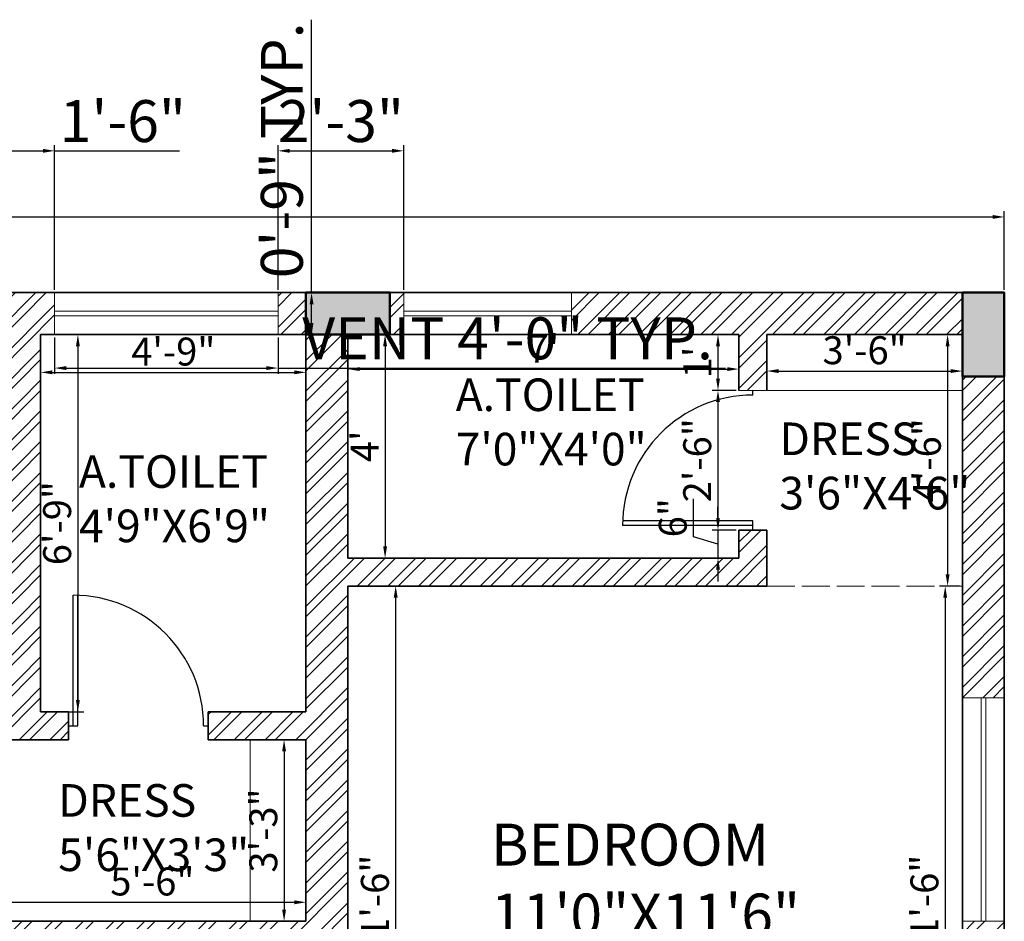
# Model space of a CAD drawing. Units: inches. Extents: x 4153 to 5577, y 785 to 1503.
# Tile 11 of 11: x 5307 to 5518, y 1309 to 1503. Entities that reach past the tile are written whole.
import ezdxf

# ---------------------------------------------------------------- set-up
doc = ezdxf.new("R2010")
doc.units = ezdxf.units.IN
doc.linetypes.add('ACAD_ISO02W100', pattern=[15, 12, -3])
for name, color, linetype, lineweight in [('A-ANNO-DIMS', 2, 'Continuous', 18), ('A-AREA-IDEN', 7, 'Continuous', 25), ('A-COLS', 7, 'Continuous', 50), ('A-DOOR', 3, 'Continuous', 25), ('A-FLOR-CASE', 32, 'Continuous', 18), ('A-GLAZ', 4, 'Continuous', 18), ('A-WALL', 7, 'Continuous', 35), ('A-WALL-OVHD', 7, 'ACAD_ISO02W100', 18)]:
    doc.layers.add(name, color=color, linetype=linetype, lineweight=lineweight)
doc.layers.add('A-WALL-PATT', color=251, linetype='Continuous', lineweight=13, true_color=0x636466)
doc.styles.get("Standard").update_dxf_attribs({"font": 'arial.ttf'})
doc.dimstyles.new('ISO-25', dxfattribs={"dimtxt": 9, "dimasz": 2.5, "dimexe": 1.25, "dimexo": 0.625, "dimtad": 1, "dimlunit": 3, "dimtxsty": 'Standard', "dimcen": 2.5, "dimadec": 0, "dimazin": 0, "dimtfac": 1, "dimtmove": 0, "dimatfit": 3, "dimfxl": 1, "dimarcsym": 0})

# ---------------------------------------------------------------- blocks, each defined once
blk = doc.blocks.new('D2')
for p, q in [((1, 0), (1, 28)), ((2, 0), (2, 27.98)), ((0, 0), (2, 0)), ((29, 0), (30, 0))]:
    blk.add_line(p, q)
at = {"ltscale": 0.5}
blk.add_arc((1, 0), 28, 0, 90, dxfattribs=at)
blk = doc.blocks.new('*D23')
at = {"layer": 'A-ANNO-DIMS', "color": 0, "lineweight": -2, "transparency": 16777216}
for p, q in [((5011.25, 1445.11), (5011.25, 1461.99)), ((5518.25, 1445.11), (5518.25, 1461.99)), ((5013.75, 1460.74), (5515.75, 1460.74))]:
    blk.add_line(p, q, dxfattribs=at)
at = {"layer": 'A-ANNO-DIMS', "color": 0, "transparency": 16777216}
for points in [[(5013.75, 1461.16), (5013.75, 1460.33), (5011.25, 1460.74)], [(5515.75, 1461.16), (5515.75, 1460.33), (5518.25, 1460.74)]]:
    blk.add_solid(points, dxfattribs=at)
at = {"layer": 'Defpoints', "color": 0, "transparency": 16777216}
for p in [(5518.25, 1460.74), (5011.25, 1444.49), (5518.25, 1444.49)]:
    blk.add_point(p, dxfattribs=at)
at = {"layer": 'A-ANNO-DIMS', "color": 0, "transparency": 16777216, "insert": (5264.75, 1465.97), "char_height": 9, "attachment_point": 5}
blk.add_mtext('42\'-3"', dxfattribs=at)
blk = doc.blocks.new('*D67')
at = {"layer": 'A-ANNO-DIMS', "color": 0, "lineweight": -2, "transparency": 16777216}
for p, q in [((5377.88, 1381.49), (5388.77, 1381.49)), ((5387.52, 1245.99), (5387.52, 1378.99)), ((5377.88, 1243.49), (5388.77, 1243.49))]:
    blk.add_line(p, q, dxfattribs=at)
at = {"layer": 'A-ANNO-DIMS', "color": 0, "transparency": 16777216}
for points in [[(5387.1, 1378.99), (5387.94, 1378.99), (5387.52, 1381.49)], [(5387.1, 1245.99), (5387.94, 1245.99), (5387.52, 1243.49)]]:
    blk.add_solid(points, dxfattribs=at)
at = {"layer": 'Defpoints', "color": 0, "transparency": 16777216}
for p in [(5377.25, 1381.49), (5387.52, 1381.49), (5377.25, 1243.49)]:
    blk.add_point(p, dxfattribs=at)
at = {"layer": 'A-ANNO-DIMS', "color": 0, "transparency": 16777216, "insert": (5383.83, 1312.49), "char_height": 6, "attachment_point": 5, "rotation": 90}
blk.add_mtext('11\'-6"', dxfattribs=at)
blk = doc.blocks.new('*D71')
at = {"layer": 'A-ANNO-DIMS', "color": 0, "lineweight": -2, "transparency": 16777216}
for p, q in [((5311.25, 1434.86), (5311.25, 1426.12)), ((5368.25, 1434.86), (5368.25, 1426.12)), ((5313.75, 1427.37), (5365.75, 1427.37))]:
    blk.add_line(p, q, dxfattribs=at)
at = {"layer": 'A-ANNO-DIMS', "color": 0, "transparency": 16777216}
for points in [[(5313.75, 1427.79), (5313.75, 1426.96), (5311.25, 1427.37)], [(5365.75, 1427.79), (5365.75, 1426.96), (5368.25, 1427.37)]]:
    blk.add_solid(points, dxfattribs=at)
at = {"layer": 'Defpoints', "color": 0, "transparency": 16777216}
for p in [(5311.25, 1435.49), (5368.25, 1435.49), (5368.25, 1427.37)]:
    blk.add_point(p, dxfattribs=at)
at = {"layer": 'A-ANNO-DIMS', "color": 0, "transparency": 16777216, "insert": (5339.75, 1431.06), "char_height": 6, "attachment_point": 5}
blk.add_mtext('4\'-9"', dxfattribs=at)
blk = doc.blocks.new('*D72')
at = {"layer": 'A-ANNO-DIMS', "color": 0, "lineweight": -2, "transparency": 16777216}
for p, q in [((5311.88, 1435.49), (5320.5, 1435.49)), ((5319.25, 1432.99), (5319.25, 1356.99)), ((5311.88, 1354.49), (5320.5, 1354.49))]:
    blk.add_line(p, q, dxfattribs=at)
at = {"layer": 'A-ANNO-DIMS', "color": 0, "transparency": 16777216}
for points in [[(5318.84, 1432.99), (5319.67, 1432.99), (5319.25, 1435.49)], [(5318.84, 1356.99), (5319.67, 1356.99), (5319.25, 1354.49)]]:
    blk.add_solid(points, dxfattribs=at)
at = {"layer": 'Defpoints', "color": 0, "transparency": 16777216}
for p in [(5311.25, 1435.49), (5311.25, 1354.49), (5319.25, 1354.49)]:
    blk.add_point(p, dxfattribs=at)
at = {"layer": 'A-ANNO-DIMS', "color": 0, "transparency": 16777216, "insert": (5315.57, 1394.99), "char_height": 6, "attachment_point": 5, "rotation": 90}
blk.add_mtext('6\'-9"', dxfattribs=at)
blk = doc.blocks.new('*D73')
at = {"layer": 'A-ANNO-DIMS', "color": 0, "lineweight": -2, "transparency": 16777216}
for p, q in [((5367.63, 1348.49), (5362.3, 1348.49)), ((5363.55, 1345.99), (5363.55, 1311.99)), ((5367.63, 1309.49), (5362.3, 1309.49))]:
    blk.add_line(p, q, dxfattribs=at)
at = {"layer": 'A-ANNO-DIMS', "color": 0, "transparency": 16777216}
for points in [[(5363.13, 1345.99), (5363.96, 1345.99), (5363.55, 1348.49)], [(5363.13, 1311.99), (5363.96, 1311.99), (5363.55, 1309.49)]]:
    blk.add_solid(points, dxfattribs=at)
at = {"layer": 'Defpoints', "color": 0, "transparency": 16777216}
for p in [(5368.25, 1348.49), (5363.55, 1309.49), (5368.25, 1309.49)]:
    blk.add_point(p, dxfattribs=at)
at = {"layer": 'A-ANNO-DIMS', "color": 0, "transparency": 16777216, "insert": (5359.86, 1328.99), "char_height": 6, "attachment_point": 5, "rotation": 90}
blk.add_mtext('3\'-3"', dxfattribs=at)
blk = doc.blocks.new('*D74')
at = {"layer": 'A-ANNO-DIMS', "color": 0, "lineweight": -2, "transparency": 16777216}
for p, q in [((5302.25, 1310.11), (5302.25, 1314.82)), ((5304.75, 1313.57), (5365.75, 1313.57)), ((5368.25, 1310.11), (5368.25, 1314.82))]:
    blk.add_line(p, q, dxfattribs=at)
at = {"layer": 'A-ANNO-DIMS', "color": 0, "transparency": 16777216}
for points in [[(5304.75, 1313.99), (5304.75, 1313.15), (5302.25, 1313.57)], [(5365.75, 1313.99), (5365.75, 1313.15), (5368.25, 1313.57)]]:
    blk.add_solid(points, dxfattribs=at)
at = {"layer": 'Defpoints', "color": 0, "transparency": 16777216}
for p in [(5368.25, 1313.57), (5302.25, 1309.49), (5368.25, 1309.49)]:
    blk.add_point(p, dxfattribs=at)
at = {"layer": 'A-ANNO-DIMS', "color": 0, "transparency": 16777216, "insert": (5335.25, 1317.26), "char_height": 6, "attachment_point": 5}
blk.add_mtext('5\'-6"', dxfattribs=at)
blk = doc.blocks.new('*D75')
at = {"layer": 'A-ANNO-DIMS', "color": 0, "lineweight": -2, "transparency": 16777216}
for p, q in [((5377.88, 1435.49), (5386.49, 1435.49)), ((5385.24, 1432.99), (5385.24, 1389.99)), ((5377.88, 1387.49), (5386.49, 1387.49))]:
    blk.add_line(p, q, dxfattribs=at)
at = {"layer": 'A-ANNO-DIMS', "color": 0, "transparency": 16777216}
for points in [[(5384.83, 1432.99), (5385.66, 1432.99), (5385.24, 1435.49)], [(5384.83, 1389.99), (5385.66, 1389.99), (5385.24, 1387.49)]]:
    blk.add_solid(points, dxfattribs=at)
at = {"layer": 'Defpoints', "color": 0, "transparency": 16777216}
for p in [(5377.25, 1435.49), (5377.25, 1387.49), (5385.24, 1387.49)]:
    blk.add_point(p, dxfattribs=at)
at = {"layer": 'A-ANNO-DIMS', "color": 0, "transparency": 16777216, "insert": (5381.62, 1411.49), "char_height": 6, "attachment_point": 5, "rotation": 90}
blk.add_mtext("4'", dxfattribs=at)
blk = doc.blocks.new('*D76')
at = {"layer": 'A-ANNO-DIMS', "color": 0, "lineweight": -2, "transparency": 16777216}
for p, q in [((5377.25, 1434.86), (5377.25, 1426.82)), ((5461.25, 1434.86), (5461.25, 1426.82)), ((5379.75, 1428.07), (5458.75, 1428.07))]:
    blk.add_line(p, q, dxfattribs=at)
at = {"layer": 'A-ANNO-DIMS', "color": 0, "transparency": 16777216}
for points in [[(5379.75, 1428.49), (5379.75, 1427.66), (5377.25, 1428.07)], [(5458.75, 1428.49), (5458.75, 1427.66), (5461.25, 1428.07)]]:
    blk.add_solid(points, dxfattribs=at)
at = {"layer": 'Defpoints', "color": 0, "transparency": 16777216}
for p in [(5377.25, 1435.49), (5461.25, 1435.49), (5461.25, 1428.07)]:
    blk.add_point(p, dxfattribs=at)
at = {"layer": 'A-ANNO-DIMS', "color": 0, "transparency": 16777216, "insert": (5419.25, 1431.7), "char_height": 6, "attachment_point": 5}
blk.add_mtext("7'", dxfattribs=at)
blk = doc.blocks.new('*D77')
at = {"layer": 'A-ANNO-DIMS', "color": 0, "lineweight": -2, "transparency": 16777216}
for p, q in [((5460.63, 1435.49), (5455.5, 1435.49)), ((5456.75, 1432.99), (5456.75, 1425.99)), ((5460.63, 1423.49), (5455.5, 1423.49))]:
    blk.add_line(p, q, dxfattribs=at)
at = {"layer": 'A-ANNO-DIMS', "color": 0, "transparency": 16777216}
for points in [[(5456.34, 1432.99), (5457.17, 1432.99), (5456.75, 1435.49)], [(5456.34, 1425.99), (5457.17, 1425.99), (5456.75, 1423.49)]]:
    blk.add_solid(points, dxfattribs=at)
at = {"layer": 'Defpoints', "color": 0, "transparency": 16777216}
for p in [(5461.25, 1435.49), (5456.75, 1423.49), (5461.25, 1423.49)]:
    blk.add_point(p, dxfattribs=at)
at = {"layer": 'A-ANNO-DIMS', "color": 0, "transparency": 16777216, "insert": (5453.12, 1429.49), "char_height": 6, "attachment_point": 5, "rotation": 90}
blk.add_mtext("1'", dxfattribs=at)
blk = doc.blocks.new('*D78')
at = {"layer": 'A-ANNO-DIMS', "color": 0, "lineweight": -2, "transparency": 16777216}
for p, q in [((5460.63, 1423.49), (5455.5, 1423.49)), ((5456.75, 1420.99), (5456.75, 1395.99)), ((5460.63, 1393.49), (5455.5, 1393.49))]:
    blk.add_line(p, q, dxfattribs=at)
at = {"layer": 'A-ANNO-DIMS', "color": 0, "transparency": 16777216}
for points in [[(5456.34, 1420.99), (5457.17, 1420.99), (5456.75, 1423.49)], [(5456.34, 1395.99), (5457.17, 1395.99), (5456.75, 1393.49)]]:
    blk.add_solid(points, dxfattribs=at)
at = {"layer": 'Defpoints', "color": 0, "transparency": 16777216}
for p in [(5461.25, 1423.49), (5456.75, 1393.49), (5461.25, 1393.49)]:
    blk.add_point(p, dxfattribs=at)
at = {"layer": 'A-ANNO-DIMS', "color": 0, "transparency": 16777216, "insert": (5453.06, 1408.49), "char_height": 6, "attachment_point": 5, "rotation": 90}
blk.add_mtext('2\'-6"', dxfattribs=at)
blk = doc.blocks.new('*D79')
at = {"layer": 'A-ANNO-DIMS', "color": 0, "lineweight": -2, "transparency": 16777216}
for p, q in [((5451.5, 1392.06), (5451.5, 1400.24)), ((5456.75, 1395.99), (5456.75, 1398.49)), ((5456.75, 1390.49), (5451.5, 1392.06)), ((5460.63, 1393.49), (5455.5, 1393.49)), ((5456.75, 1393.49), (5456.75, 1387.49)), ((5456.75, 1393.49), (5456.75, 1387.49)), ((5460.63, 1387.49), (5455.5, 1387.49)), ((5456.75, 1384.99), (5456.75, 1382.49))]:
    blk.add_line(p, q, dxfattribs=at)
at = {"layer": 'A-ANNO-DIMS', "color": 0, "transparency": 16777216}
for points in [[(5456.34, 1395.99), (5457.17, 1395.99), (5456.75, 1393.49)], [(5456.34, 1384.99), (5457.17, 1384.99), (5456.75, 1387.49)]]:
    blk.add_solid(points, dxfattribs=at)
at = {"layer": 'Defpoints', "color": 0, "transparency": 16777216}
for p in [(5461.25, 1393.49), (5456.75, 1387.49), (5461.25, 1387.49)]:
    blk.add_point(p, dxfattribs=at)
at = {"layer": 'A-ANNO-DIMS', "color": 0, "transparency": 16777216, "insert": (5447.81, 1396.15), "char_height": 6, "attachment_point": 5, "rotation": 90}
blk.add_mtext('6"', dxfattribs=at)
blk = doc.blocks.new('*D80')
at = {"layer": 'A-ANNO-DIMS', "color": 0, "lineweight": -2, "transparency": 16777216}
for p, q in [((5467.25, 1434.86), (5467.25, 1426.39)), ((5509.25, 1434.86), (5509.25, 1426.39)), ((5469.75, 1427.64), (5506.75, 1427.64))]:
    blk.add_line(p, q, dxfattribs=at)
at = {"layer": 'A-ANNO-DIMS', "color": 0, "transparency": 16777216}
for points in [[(5469.75, 1428.06), (5469.75, 1427.23), (5467.25, 1427.64)], [(5506.75, 1428.06), (5506.75, 1427.23), (5509.25, 1427.64)]]:
    blk.add_solid(points, dxfattribs=at)
at = {"layer": 'Defpoints', "color": 0, "transparency": 16777216}
for p in [(5467.25, 1435.49), (5509.25, 1435.49), (5509.25, 1427.64)]:
    blk.add_point(p, dxfattribs=at)
at = {"layer": 'A-ANNO-DIMS', "color": 0, "transparency": 16777216, "insert": (5488.25, 1431.34), "char_height": 6, "attachment_point": 5}
blk.add_mtext('3\'-6"', dxfattribs=at)
blk = doc.blocks.new('*D81')
at = {"layer": 'A-ANNO-DIMS', "color": 0, "lineweight": -2, "transparency": 16777216}
for p, q in [((5508.63, 1435.49), (5504.82, 1435.49)), ((5506.07, 1432.99), (5506.07, 1383.99)), ((5508.63, 1381.49), (5504.82, 1381.49))]:
    blk.add_line(p, q, dxfattribs=at)
at = {"layer": 'A-ANNO-DIMS', "color": 0, "transparency": 16777216}
for points in [[(5505.66, 1432.99), (5506.49, 1432.99), (5506.07, 1435.49)], [(5505.66, 1383.99), (5506.49, 1383.99), (5506.07, 1381.49)]]:
    blk.add_solid(points, dxfattribs=at)
at = {"layer": 'Defpoints', "color": 0, "transparency": 16777216}
for p in [(5509.25, 1435.49), (5506.07, 1381.49), (5509.25, 1381.49)]:
    blk.add_point(p, dxfattribs=at)
at = {"layer": 'A-ANNO-DIMS', "color": 0, "transparency": 16777216, "insert": (5502.39, 1408.49), "char_height": 6, "attachment_point": 5, "rotation": 90}
blk.add_mtext('4\'-6"', dxfattribs=at)
blk = doc.blocks.new('*D82')
at = {"layer": 'A-ANNO-DIMS', "color": 0, "lineweight": -2, "transparency": 16777216}
for p, q in [((5508.63, 1381.49), (5504.31, 1381.49)), ((5505.56, 1378.99), (5505.56, 1245.99)), ((5508.63, 1243.49), (5504.31, 1243.49))]:
    blk.add_line(p, q, dxfattribs=at)
at = {"layer": 'A-ANNO-DIMS', "color": 0, "transparency": 16777216}
for points in [[(5505.14, 1378.99), (5505.97, 1378.99), (5505.56, 1381.49)], [(5505.14, 1245.99), (5505.97, 1245.99), (5505.56, 1243.49)]]:
    blk.add_solid(points, dxfattribs=at)
at = {"layer": 'Defpoints', "color": 0, "transparency": 16777216}
for p in [(5509.25, 1381.49), (5505.56, 1243.49), (5509.25, 1243.49)]:
    blk.add_point(p, dxfattribs=at)
at = {"layer": 'A-ANNO-DIMS', "color": 0, "transparency": 16777216, "insert": (5501.87, 1312.49), "char_height": 6, "attachment_point": 5, "rotation": 90}
blk.add_mtext('11\'-6"', dxfattribs=at)
blk = doc.blocks.new('WINDOW-48IN')
for p, q in [((0, 9), (0, 0)), ((48, 9), (48, 0)), ((0, 5), (48, 5)), ((0, 4), (48, 4))]:
    blk.add_line(p, q)
blk = doc.blocks.new('VENT-WINDOW-48IN')
for p, q in [((0, 9), (0, 0)), ((48, 9), (48, 0)), ((0, 5), (48, 5)), ((0, 4), (48, 4))]:
    blk.add_line(p, q)
blk = doc.blocks.new('VENT-WINDOW-36IN')
for p, q in [((0, 9), (0, 0)), ((36, 9), (36, 0)), ((0, 5), (36, 5)), ((0, 4), (36, 4))]:
    blk.add_line(p, q)
blk = doc.blocks.new('COL-9X18IN')
at = {"transparency": 33554687}
h = blk.add_hatch(color=256, dxfattribs=at)
h.dxf.hatch_style = 1
h.paths.add_polyline_path([(9, 18), (0, 18), (0, 0), (9, 0)])
blk.add_lwpolyline([(0, 18), (9, 18), (9, 0), (0, 0)], close=True)
blk = doc.blocks.new('*D106')
at = {"layer": 'A-ANNO-DIMS', "color": 0, "lineweight": -2, "transparency": 16777216}
for p, q in [((5314.25, 1434.86), (5314.25, 1427.04)), ((5362.25, 1434.86), (5362.25, 1427.04)), ((5316.75, 1428.29), (5359.75, 1428.29)), ((5362.25, 1428.29), (5458.36, 1428.29))]:
    blk.add_line(p, q, dxfattribs=at)
at = {"layer": 'A-ANNO-DIMS', "color": 0, "transparency": 16777216}
for points in [[(5316.75, 1428.71), (5316.75, 1427.87), (5314.25, 1428.29)], [(5359.75, 1428.71), (5359.75, 1427.87), (5362.25, 1428.29)]]:
    blk.add_solid(points, dxfattribs=at)
at = {"layer": 'Defpoints', "color": 0, "transparency": 16777216}
for p in [(5314.25, 1435.49), (5362.25, 1435.49), (5362.25, 1428.29)]:
    blk.add_point(p, dxfattribs=at)
at = {"layer": 'A-ANNO-DIMS', "color": 0, "transparency": 16777216, "insert": (5411.55, 1433.51), "char_height": 9, "attachment_point": 5}
blk.add_mtext('VENT 4\'-0" TYP.', dxfattribs=at)
blk = doc.blocks.new('*D107')
at = {"layer": 'A-ANNO-DIMS', "color": 0, "lineweight": -2, "transparency": 16777216}
for p, q in [((5369.45, 1444.49), (5369.45, 1503.1)), ((5362.88, 1444.49), (5370.7, 1444.49)), ((5369.45, 1437.99), (5369.45, 1441.99)), ((5362.88, 1435.49), (5370.7, 1435.49))]:
    blk.add_line(p, q, dxfattribs=at)
at = {"layer": 'A-ANNO-DIMS', "color": 0, "transparency": 16777216}
for points in [[(5369.04, 1441.99), (5369.87, 1441.99), (5369.45, 1444.49)], [(5369.04, 1437.99), (5369.87, 1437.99), (5369.45, 1435.49)]]:
    blk.add_solid(points, dxfattribs=at)
at = {"layer": 'Defpoints', "color": 0, "transparency": 16777216}
for p in [(5362.25, 1444.49), (5369.45, 1444.49), (5362.25, 1435.49)]:
    blk.add_point(p, dxfattribs=at)
at = {"layer": 'A-ANNO-DIMS', "color": 0, "transparency": 16777216, "insert": (5364.23, 1475.04), "char_height": 9, "attachment_point": 5, "rotation": 90}
blk.add_mtext('0\'-9" TYP.', dxfattribs=at)
blk = doc.blocks.new('*D148')
at = {"layer": 'A-ANNO-DIMS', "color": 0, "lineweight": -2, "transparency": 16777216}
for p, q in [((5296.25, 1445.11), (5296.25, 1476.19)), ((5298.75, 1474.94), (5311.75, 1474.94)), ((5314.25, 1445.11), (5314.25, 1476.19)), ((5314.25, 1474.94), (5341.08, 1474.94))]:
    blk.add_line(p, q, dxfattribs=at)
at = {"layer": 'A-ANNO-DIMS', "color": 0, "transparency": 16777216}
for points in [[(5298.75, 1475.36), (5298.75, 1474.52), (5296.25, 1474.94)], [(5311.75, 1475.36), (5311.75, 1474.52), (5314.25, 1474.94)]]:
    blk.add_solid(points, dxfattribs=at)
at = {"layer": 'Defpoints', "color": 0, "transparency": 16777216}
for p in [(5314.25, 1474.94), (5296.25, 1444.49), (5314.25, 1444.49)]:
    blk.add_point(p, dxfattribs=at)
at = {"layer": 'A-ANNO-DIMS', "color": 0, "transparency": 16777216, "insert": (5328.92, 1480.16), "char_height": 9, "attachment_point": 5}
blk.add_mtext('1\'-6"', dxfattribs=at)
blk = doc.blocks.new('*D149')
at = {"layer": 'A-ANNO-DIMS', "color": 0, "lineweight": -2, "transparency": 16777216}
for p, q in [((5362.25, 1445.11), (5362.25, 1476.19)), ((5364.75, 1474.94), (5386.75, 1474.94)), ((5389.25, 1445.11), (5389.25, 1476.19))]:
    blk.add_line(p, q, dxfattribs=at)
at = {"layer": 'A-ANNO-DIMS', "color": 0, "transparency": 16777216}
for points in [[(5364.75, 1475.36), (5364.75, 1474.52), (5362.25, 1474.94)], [(5386.75, 1475.36), (5386.75, 1474.52), (5389.25, 1474.94)]]:
    blk.add_solid(points, dxfattribs=at)
at = {"layer": 'Defpoints', "color": 0, "transparency": 16777216}
for p in [(5389.25, 1474.94), (5362.25, 1444.49), (5389.25, 1444.49)]:
    blk.add_point(p, dxfattribs=at)
at = {"layer": 'A-ANNO-DIMS', "color": 0, "transparency": 16777216, "insert": (5375.75, 1480.16), "char_height": 9, "attachment_point": 5}
blk.add_mtext('2\'-3"', dxfattribs=at)

msp = doc.modelspace()

# ---------------------------------------------------------------- hatches: boundary and pattern name
at = {"layer": 'A-WALL-PATT', "transparency": 33554687}
h = msp.add_hatch(dxfattribs=at)
h.set_pattern_fill('ANSI32', color=256, scale=0.49)
h.set_pattern_definition([(45, (816.3263, 0), (-3.300244, 3.300244), []), (45, (818.5265, 0), (-3.300244, 3.300244), [])])
h.paths.add_polyline_path([(5011.254, 1088.988), (5020.254, 1088.988), (5020.254, 1129.488), (5155.254, 1129.488), (5155.254, 1105.488), (5161.254, 1105.488), (5161.254, 1138.488), (5098.254, 1138.488), (5098.254, 1234.488), (5113.254, 1234.488), (5113.254, 1243.488), (5086.254, 1243.488), (5086.254, 1234.488), (5092.254, 1234.488), (5092.254, 1138.488), (5020.254, 1138.488), (5020.254, 1168.488), (5011.254, 1168.488)])
h.paths.add_polyline_path([(5011.254, 1009.488), (5020.254, 1009.488), (5020.254, 1040.988), (5011.254, 1040.988)])
h.paths.add_polyline_path([(5095.254, 991.488), (5095.254, 1000.488), (5020.254, 1000.488), (5020.254, 991.488)])
h.paths.add_polyline_path([(5011.254, 910.488), (5020.254, 910.488), (5020.254, 991.488), (5011.254, 991.488)])
h.paths.add_polyline_path([(5152.254, 901.488), (5152.254, 907.488), (5020.254, 907.488), (5020.254, 901.488)])
h.paths.add_polyline_path([(5161.254, 1057.488), (5155.254, 1057.488), (5155.254, 1000.488), (5161.254, 1000.488)])
h.paths.add_polyline_path([(5143.254, 991.488), (5152.254, 991.488), (5152.254, 1000.488), (5143.254, 1000.488)])
h.paths.add_polyline_path([(5161.254, 1000.488), (5161.254, 991.488), (5185.254, 991.488), (5185.254, 1000.488)])
h.paths.add_polyline_path([(5257.254, 991.488), (5257.254, 1000.488), (5233.254, 1000.488), (5233.254, 991.488)])
h.paths.add_polyline_path([(5266.254, 1120.488), (5257.254, 1120.488), (5257.254, 1000.488), (5266.254, 1000.488)])
h.paths.add_polyline_path([(5290.254, 991.488), (5290.254, 1000.488), (5275.254, 1000.488), (5275.254, 991.488)])
h.paths.add_polyline_path([(5362.254, 1000.488), (5362.254, 991.488), (5455.254, 991.488), (5455.254, 1000.488)])
h.paths.add_polyline_path([(5509.254, 1009.488), (5518.254, 1009.488), (5518.254, 1036.488), (5509.254, 1036.488)])
h.paths.add_polyline_path([(5503.254, 1000.488), (5503.254, 991.488), (5509.254, 991.488), (5509.254, 1000.488)])
h.paths.add_polyline_path([(5518.254, 1132.488), (5509.254, 1132.488), (5509.254, 1108.488), (5518.254, 1108.488)])
h.paths.add_polyline_path([(5509.254, 1204.488), (5518.254, 1204.488), (5518.254, 1225.488), (5509.254, 1225.488)])
h.paths.add_polyline_path([(5467.254, 1234.488), (5467.254, 1243.488), (5377.254, 1243.488), (5377.254, 1265.228), (5377.254, 1381.488), (5467.254, 1381.488), (5467.254, 1393.488), (5461.254, 1393.488), (5461.254, 1387.488), (5377.254, 1387.488), (5377.254, 1435.488), (5368.254, 1435.488), (5368.254, 1354.488), (5347.254, 1354.488), (5347.254, 1348.488), (5368.254, 1348.488), (5368.254, 1309.488), (5302.254, 1309.488), (5302.254, 1234.488), (5321.754, 1234.488), (5321.754, 1243.488), (5311.254, 1243.488), (5311.254, 1303.488), (5368.254, 1303.488), (5368.254, 1243.488), (5357.754, 1243.488), (5357.754, 1234.488)])
h.paths.add_polyline_path([(5509.254, 1357.488), (5518.254, 1357.488), (5518.254, 1426.488), (5509.254, 1426.488)])
h.paths.add_polyline_path([(5509.254, 1243.488), (5518.254, 1243.488), (5518.254, 1309.488), (5509.254, 1309.488)])
h.paths.add_polyline_path([(5509.254, 1435.488), (5509.254, 1444.488), (5425.254, 1444.488), (5425.254, 1435.488), (5461.254, 1435.488), (5461.254, 1423.488), (5467.254, 1423.488), (5467.254, 1435.488)])
h.paths.add_polyline_path([(5302.254, 1435.488), (5302.254, 1348.488), (5317.254, 1348.488), (5317.254, 1354.488), (5311.254, 1354.488), (5311.254, 1435.488), (5314.254, 1435.488), (5314.254, 1444.488), (5296.254, 1444.488), (5296.254, 1435.488)])
h.paths.add_polyline_path([(5368.254, 1444.488), (5362.254, 1444.488), (5362.254, 1435.488), (5368.254, 1435.488)])
h.paths.add_polyline_path([(5389.254, 1444.488), (5386.254, 1444.488), (5386.254, 1435.488), (5389.254, 1435.488)])
h.paths.add_polyline_path([(5248.254, 1435.488), (5248.254, 1444.488), (5173.254, 1444.488), (5173.254, 1435.488)])
h.paths.add_polyline_path([(5101.254, 1435.488), (5101.254, 1444.488), (5020.254, 1444.488), (5020.254, 1435.488)])
h.paths.add_polyline_path([(5011.254, 1293.488), (5020.254, 1293.488), (5020.254, 1295.242), (5020.254, 1426.488), (5011.254, 1426.488)])
h.paths.add_polyline_path([(5155.254, 1243.488), (5149.254, 1243.488), (5149.254, 1234.488), (5248.254, 1234.488), (5248.254, 1243.488), (5164.254, 1243.488), (5164.254, 1435.488), (5155.254, 1435.488)])
h.paths.add_polyline_path([(5020.254, 1243.488), (5020.254, 1234.488), (5056.254, 1234.488), (5056.254, 1243.488)], flags=17)
h.paths.add_polyline_path([(5020.254, 1225.488), (5011.254, 1225.488), (5011.254, 1198.488), (5020.254, 1198.488)], flags=17)

# ---------------------------------------------------------------- linework, layer by layer
at = {"layer": 'A-FLOR-CASE'}
for p, q in [((5461.254, 1423.488), (5509.254, 1423.488)), ((5356.254, 1309.488), (5356.254, 1348.488))]:
    msp.add_line(p, q, dxfattribs=at)
at = {"layer": 'A-WALL'}
for p, q in [((5011.254, 1444.488), (5518.254, 1444.488)), ((5518.254, 1444.488), (5518.254, 901.488)), ((5311.254, 1435.488), (5368.254, 1435.488)), ((5311.254, 1354.488), (5311.254, 1435.488)), ((5368.254, 1354.488), (5368.254, 1435.488)), ((5377.254, 1435.488), (5461.254, 1435.488)), ((5377.254, 1387.488), (5377.254, 1435.488)), ((5461.254, 1423.488), (5461.254, 1435.488)), ((5467.254, 1435.488), (5509.254, 1435.488)), ((5467.254, 1423.488), (5467.254, 1435.488)), ((5509.254, 1435.488), (5509.254, 1243.488)), ((5461.254, 1393.488), (5467.254, 1393.488)), ((5461.254, 1387.488), (5461.254, 1393.488)), ((5467.254, 1393.488), (5467.254, 1381.488)), ((5377.254, 1387.488), (5461.254, 1387.488)), ((5377.254, 1381.488), (5467.254, 1381.488)), ((5377.254, 1243.488), (5377.254, 1381.488)), ((5311.254, 1354.488), (5317.254, 1354.488)), ((5317.254, 1348.488), (5317.254, 1354.488)), ((5347.254, 1354.488), (5368.254, 1354.488)), ((5347.254, 1348.488), (5347.254, 1354.488)), ((5302.254, 1348.488), (5317.254, 1348.488)), ((5347.254, 1348.488), (5368.254, 1348.488)), ((5368.254, 1309.488), (5368.254, 1348.488)), ((5302.254, 1309.488), (5368.254, 1309.488))]:
    msp.add_line(p, q, dxfattribs=at)
at = {"layer": 'A-WALL-OVHD', "ltscale": 0.5}
msp.add_line((5467.254, 1381.488), (5509.254, 1381.488), dxfattribs=at)

# ---------------------------------------------------------------- block references
at = {"layer": 'A-COLS', "rotation": 270.0000000000022}
msp.add_blockref('COL-9X18IN', (5368.254, 1444.488), dxfattribs=at)
at = {"layer": 'A-COLS'}
msp.add_blockref('COL-9X18IN', (5509.254, 1426.488), dxfattribs=at)
at = {"layer": 'A-DOOR', "rotation": 90}
msp.add_blockref('D2', (5464.254, 1393.488), dxfattribs=at)
at = {"layer": 'A-DOOR'}
msp.add_blockref('D2', (5317.254, 1351.488), dxfattribs=at)
at = {"layer": 'A-GLAZ'}
for name, p in [('VENT-WINDOW-48IN', (5314.254, 1435.488)), ('VENT-WINDOW-36IN', (5389.254, 1435.488))]:
    msp.add_blockref(name, p, dxfattribs=at)
at = {"layer": 'A-GLAZ', "rotation": 270.0000000000016}
msp.add_blockref('WINDOW-48IN', (5509.254, 1357.488), dxfattribs=at)

# ---------------------------------------------------------------- texts
at = {"layer": 'A-AREA-IDEN', "attachment_point": 1}
for s, heights, insert, char_height in [('{\\fTimes New Roman|b0|i0|c0|p18;A.TOILET\\P7\'0"X4\'0"}', [0], (5400.408, 1426.054), 7), ('{\\fTimes New Roman|b0|i0|c0|p18;DRESS\\P3\'6"X4\'6"}', [0], (5469.932, 1416.602), 7), ('{\\fTimes New Roman|b0|i0|c0|p18;A.TOILET\\P4\'9"X6\'9"}', [18.808], (5319.482, 1409.571), 7), ('{\\fTimes New Roman|b0|i0|c0|p18;DRESS\\P5\'6"X3\'3"}', [18.808], (5315.033, 1338.946), 7), ('{\\fTimes New Roman|b0|i0|c0|p18;BEDROOM\\P11\'0"X11\'6"}', [0], (5407.994, 1330.447), 9)]:
    msp.add_mtext_dynamic_manual_height_columns(s, width=67.35079, gutter_width=12.5, heights=heights, dxfattribs=dict(at, insert=insert, char_height=char_height))

# ---------------------------------------------------------------- dimensions: what is measured, and where the dimension line sits
at = {"layer": 'A-ANNO-DIMS'}
dim = msp.add_linear_dim(base=(5369.454, 1444.488), p1=(5362.254, 1435.488), p2=(5362.254, 1444.488), angle=90, text='<> TYP.', dimstyle='ISO-25', override={"dimdec": 1, "dimlfac": 1, "dimrnd": 0, "dimzin": 1, "dimdsep": 46, "dimlunit": 4, "dimfrac": 2}, dxfattribs=at)
dim.commit()
dim.dimension.update_dxf_attribs({"geometry": '*D107', "text_midpoint": (5364.234, 1475.043)})
for base, p1, p2, override, picture, middle in [((5314.254, 1474.938), (5296.254, 1444.488), (5314.254, 1444.488), {"dimdec": 1, "dimlfac": 1, "dimrnd": 0, "dimzin": 1, "dimdsep": 46, "dimlunit": 4, "dimfrac": 2}, '*D148', (5328.917, 1480.159)), ((5389.254, 1474.938), (5362.254, 1444.488), (5389.254, 1444.488), {"dimdec": 1, "dimlfac": 1, "dimrnd": 0, "dimzin": 1, "dimdsep": 46, "dimlunit": 4, "dimfrac": 2}, '*D149', (5375.754, 1480.162)), ((5518.254, 1460.744), (5011.254, 1444.488), (5518.254, 1444.488), {"dimclrd": 0, "dimclre": 0, "dimclrt": 0}, '*D23', (5264.754, 1465.968)), ((5368.254, 1427.372), (5311.254, 1435.488), (5368.254, 1435.488), {"dimtxt": 6, "dimclrd": 0, "dimclre": 0, "dimclrt": 0}, '*D71', (5339.754, 1431.061)), ((5461.254, 1428.072), (5377.254, 1435.488), (5461.254, 1435.488), {"dimtxt": 6, "dimclrd": 0, "dimclre": 0, "dimclrt": 0}, '*D76', (5419.254, 1431.697)), ((5509.254, 1427.645), (5467.254, 1435.488), (5509.254, 1435.488), {"dimtxt": 6, "dimclrd": 0, "dimclre": 0, "dimclrt": 0}, '*D80', (5488.254, 1431.335)), ((5368.254, 1313.571), (5302.254, 1309.488), (5368.254, 1309.488), {"dimtxt": 6, "dimclrd": 0, "dimclre": 0, "dimclrt": 0}, '*D74', (5335.254, 1317.26))]:
    dim = msp.add_linear_dim(base=base, p1=p1, p2=p2, dimstyle='ISO-25', override=override, dxfattribs=at)
    dim.commit()
    dim.dimension.update_dxf_attribs({"geometry": picture, "text_midpoint": middle})
dim = msp.add_linear_dim(base=(5362.254, 1428.288), p1=(5314.254, 1435.488), p2=(5362.254, 1435.488), text='VENT <> TYP.', dimstyle='ISO-25', override={"dimdec": 1, "dimlfac": 1, "dimrnd": 0, "dimzin": 1, "dimdsep": 46, "dimlunit": 4, "dimfrac": 2}, dxfattribs=at)
dim.commit()
dim.dimension.update_dxf_attribs({"geometry": '*D106', "text_midpoint": (5411.554, 1433.509)})
for base, p1, p2, override, picture, middle in [((5319.254, 1354.488), (5311.254, 1435.488), (5311.254, 1354.488), {"dimtxt": 6, "dimclrd": 0, "dimclre": 0, "dimclrt": 0}, '*D72', (5315.565, 1394.988)), ((5385.244, 1387.488), (5377.254, 1435.488), (5377.254, 1387.488), {"dimtxt": 6, "dimclrd": 0, "dimclre": 0, "dimclrt": 0}, '*D75', (5381.619, 1411.488)), ((5456.752, 1423.488), (5461.254, 1435.488), (5461.254, 1423.488), {"dimtxt": 6, "dimclrd": 0, "dimclre": 0, "dimclrt": 0}, '*D77', (5453.115, 1429.488)), ((5506.075, 1381.488), (5509.254, 1435.488), (5509.254, 1381.488), {"dimtxt": 6, "dimclrd": 0, "dimclre": 0, "dimclrt": 0}, '*D81', (5502.386, 1408.488)), ((5456.752, 1393.488), (5461.254, 1423.488), (5461.254, 1393.488), {"dimtxt": 6, "dimclrd": 0, "dimclre": 0, "dimclrt": 0, "dimtmove": 1}, '*D78', (5453.064, 1408.488)), ((5456.752, 1387.488), (5461.254, 1393.488), (5461.254, 1387.488), {"dimtxt": 6, "dimclrd": 0, "dimclre": 0, "dimclrt": 0, "dimtmove": 1}, '*D79', (5447.813, 1392.689)), ((5387.52, 1381.488), (5377.254, 1243.488), (5377.254, 1381.488), {"dimtxt": 6, "dimclrd": 0, "dimclre": 0, "dimclrt": 0}, '*D67', (5383.832, 1312.488)), ((5505.555, 1243.488), (5509.254, 1381.488), (5509.254, 1243.488), {"dimtxt": 6, "dimclrd": 0, "dimclre": 0, "dimclrt": 0}, '*D82', (5501.867, 1312.488)), ((5363.547, 1309.488), (5368.254, 1348.488), (5368.254, 1309.488), {"dimtxt": 6, "dimclrd": 0, "dimclre": 0, "dimclrt": 0}, '*D73', (5359.857, 1328.988))]:
    dim = msp.add_linear_dim(base=base, p1=p1, p2=p2, angle=90, dimstyle='ISO-25', override=override, dxfattribs=at)
    dim.commit()
    dim.dimension.update_dxf_attribs({"geometry": picture, "text_midpoint": middle})

doc.saveas('drawing.dxf')
